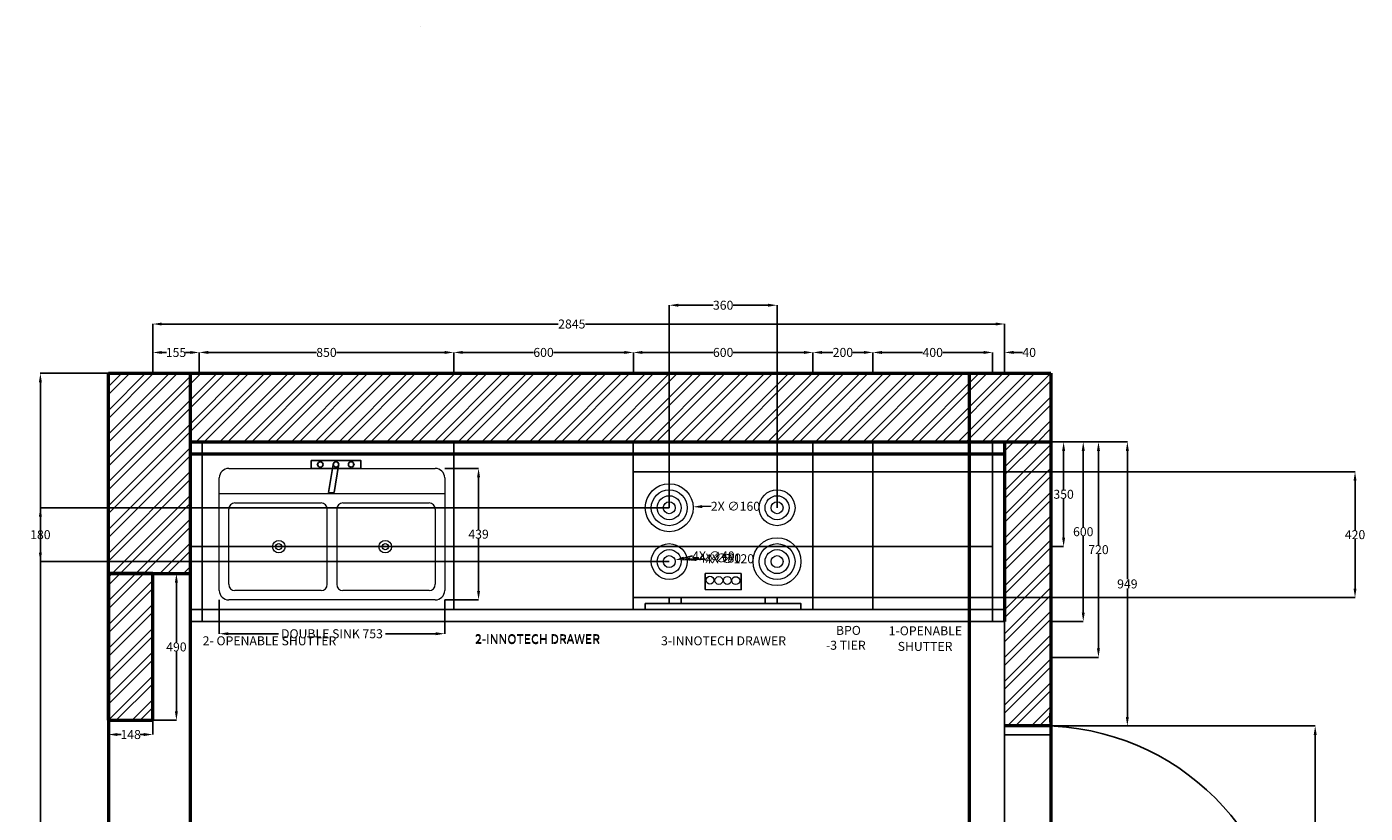
# Model space of a CAD drawing. Units: millimetres. Extents: x 26138 to 44889, y 15820 to 21179.
# Tile 2 of 8: x 26144 to 30614, y 18552 to 21179. Entities that reach past the tile are written whole.
import ezdxf

# ---------------------------------------------------------------- set-up
doc = ezdxf.new("R2010")
doc.units = ezdxf.units.MM
doc.header["$MEASUREMENT"] = 0
doc.header["$PDMODE"] = 3
for name, color, linetype, lineweight in [('A-ANNO-DIMS', 70, 'Continuous', 18), ('A-ANNO-TEXT', 7, 'Continuous', 18), ('A-DOOR', 4, 'Continuous', 25), ('A-EQPM', 8, 'Continuous', 18), ('A-FLOR-FIXT', 8, 'Continuous', 18), ('A-FURN', 26, 'Continuous', 25), ('A-WALL', 1, 'Continuous', 50), ('A-WALL-PATT', 8, 'Continuous', 13)]:
    doc.layers.add(name, color=color, linetype=linetype, lineweight=lineweight)
doc.styles.get("Standard").update_dxf_attribs({"font": 'arial.ttf'})
doc.dimstyles.get("Standard").update_dxf_attribs({"dimtxt": 30, "dimasz": 30, "dimexe": 0.18, "dimexo": 0.0625, "dimgap": 0.09, "dimtad": 0, "dimtih": 1, "dimtoh": 1, "dimdec": 0, "dimzin": 0, "dimdsep": 46, "dimtxsty": 'Standard', "dimcen": 0.09, "dimadec": 0, "dimazin": 0, "dimtfac": 1, "dimtdec": 0, "dimtofl": 0, "dimtmove": 0, "dimatfit": 3, "dimfxl": 1, "dimtolj": 1, "dimtzin": 0, "dimarcsym": 0})
pattern_1 = [(45, (-272.624, -1462.17), (-39.77476, 39.77476), []), (45, (-246.11, -1462.17), (-39.77476, 39.77476), [])]

# ---------------------------------------------------------------- blocks, each defined once
blk = doc.blocks.new('Sink-double - 36 in top')
for p, q in [((-18, -4), (18, -4)), ((-0.75, -18.5), (-0.75, -6.5)), ((0.75, -6.5), (0.75, -18.5))]:
    blk.add_line(p, q)
for points in [[(-16.5, 0), (16.5, 0)], [(-18, -19.5), (-18, -1.5)], [(18, -1.5), (18, -19.5)], [(-15.5, -5.5), (-1.75, -5.5)], [(1.75, -5.5), (15.5, -5.5)], [(-16.5, -18.5), (-16.5, -6.5)], [(16.5, -6.5), (16.5, -18.5)], [(16.5, -21), (-16.5, -21)], [(-1.75, -19.5), (-15.5, -19.5)], [(15.5, -19.5), (1.75, -19.5)]]:
    blk.add_lwpolyline(points)
for centre, radius in [((-8.5, -12.5), 1), ((-8.5, -12.5), 0.5), ((8.5, -12.5), 1), ((8.5, -12.5), 0.5)]:
    blk.add_circle(centre, radius)
for centre, radius, start, end in [((-16.5, -1.5), 1.5, 90, 180), ((16.5, -1.5), 1.5, 0, 90), ((-15.5, -6.5), 1, 90, 180), ((-1.75, -6.5), 1, 0, 90), ((1.75, -6.5), 1, 90, 180), ((15.5, -6.5), 1, 0, 90), ((-15.5, -18.5), 1, 180, 270), ((-1.75, -18.5), 1, 270, 0), ((1.75, -18.5), 1, 180, 270), ((15.5, -18.5), 1, 270, 0), ((-16.5, -19.5), 1.5, 180, 270), ((16.5, -19.5), 1.5, 270, 0)]:
    blk.add_arc(centre, radius, start, end)
blk = doc.blocks.new('*U4')
for p, q in [((0, 0), (0, -6)), ((40, 0), (40, -6))]:
    blk.add_line(p, q)
blk.add_lwpolyline([(0, 0), (0, 40), (1.75, 40), (1.75, 0)], close=True)
blk.add_arc((0, 0), 40, 0, 90)
blk = doc.blocks.new('*D5')
at = {"layer": 'A-ANNO-DIMS', "color": 0, "lineweight": -2, "transparency": 16777216}
for p, q in [((26564.5, 20021.3), (26564.5, 20186.1)), ((26594.5, 20185.9), (27918.7, 20185.9)), ((29379.5, 20185.9), (28009.2, 20185.9)), ((29409.5, 20021.3), (29409.5, 20186.1))]:
    blk.add_line(p, q, dxfattribs=at)
at = {"layer": 'A-ANNO-DIMS', "color": 0, "transparency": 16777216}
for points in [[(26594.5, 20190.9), (26594.5, 20180.9), (26564.5, 20185.9)], [(29379.5, 20190.9), (29379.5, 20180.9), (29409.5, 20185.9)]]:
    blk.add_solid(points, dxfattribs=at)
at = {"layer": 'Defpoints', "color": 0, "transparency": 16777216}
for p in [(29409.5, 20185.9), (26564.5, 20021.2), (29409.5, 20021.2)]:
    blk.add_point(p, dxfattribs=at)
at = {"layer": 'A-ANNO-DIMS', "color": 0, "transparency": 16777216, "insert": (27964, 20185.9), "char_height": 30, "attachment_point": 5}
blk.add_mtext('\\A1;2845', dxfattribs=at)
blk = doc.blocks.new('*D6')
at = {"layer": 'A-ANNO-DIMS', "color": 0, "lineweight": -2, "transparency": 16777216}
for p, q in [((26564.5, 19352.2), (26643.5, 19352.2)), ((26643.3, 19322.2), (26643.3, 19122.6)), ((26643.3, 18892.2), (26643.3, 19091.8)), ((26564.5, 18862.2), (26643.5, 18862.2))]:
    blk.add_line(p, q, dxfattribs=at)
at = {"layer": 'A-ANNO-DIMS', "color": 0, "transparency": 16777216}
for points in [[(26638.3, 19322.2), (26648.3, 19322.2), (26643.3, 19352.2)], [(26638.3, 18892.2), (26648.3, 18892.2), (26643.3, 18862.2)]]:
    blk.add_solid(points, dxfattribs=at)
at = {"layer": 'Defpoints', "color": 0, "transparency": 16777216}
for p in [(26564.5, 19352.2), (26643.3, 19352.2), (26564.5, 18862.2)]:
    blk.add_point(p, dxfattribs=at)
at = {"layer": 'A-ANNO-DIMS', "color": 0, "transparency": 16777216, "insert": (26643.3, 19107.2), "char_height": 30, "attachment_point": 5}
blk.add_mtext('\\A1;490', dxfattribs=at)
blk = doc.blocks.new('*D7')
at = {"layer": 'A-ANNO-DIMS', "color": 0, "lineweight": -2, "transparency": 16777216}
for p, q in [((29564.5, 19792.2), (29606.7, 19792.2)), ((29606.6, 19762.2), (29606.6, 19632.6)), ((29606.6, 19472.2), (29606.6, 19601.8)), ((29564.5, 19442.2), (29606.7, 19442.2))]:
    blk.add_line(p, q, dxfattribs=at)
at = {"layer": 'A-ANNO-DIMS', "color": 0, "transparency": 16777216}
for points in [[(29601.6, 19762.2), (29611.6, 19762.2), (29606.6, 19792.2)], [(29601.6, 19472.2), (29611.6, 19472.2), (29606.6, 19442.2)]]:
    blk.add_solid(points, dxfattribs=at)
at = {"layer": 'Defpoints', "color": 0, "transparency": 16777216}
for p in [(29564.5, 19792.2), (29564.5, 19442.2), (29606.6, 19442.2)]:
    blk.add_point(p, dxfattribs=at)
at = {"layer": 'A-ANNO-DIMS', "color": 0, "transparency": 16777216, "insert": (29606.6, 19617.2), "char_height": 30, "attachment_point": 5}
blk.add_mtext('\\A1;350', dxfattribs=at)
blk = doc.blocks.new('*D8')
at = {"layer": 'A-ANNO-DIMS', "color": 0, "lineweight": -2, "transparency": 16777216}
for p, q in [((29564.5, 19792.2), (29672.4, 19792.2)), ((29672.2, 19762.2), (29672.2, 19507.6)), ((29672.2, 19222.2), (29672.2, 19476.8)), ((29564.5, 19192.2), (29672.4, 19192.2))]:
    blk.add_line(p, q, dxfattribs=at)
at = {"layer": 'A-ANNO-DIMS', "color": 0, "transparency": 16777216}
for points in [[(29667.2, 19762.2), (29677.2, 19762.2), (29672.2, 19792.2)], [(29667.2, 19222.2), (29677.2, 19222.2), (29672.2, 19192.2)]]:
    blk.add_solid(points, dxfattribs=at)
at = {"layer": 'Defpoints', "color": 0, "transparency": 16777216}
for p in [(29564.5, 19792.2), (29564.5, 19192.2), (29672.2, 19192.2)]:
    blk.add_point(p, dxfattribs=at)
at = {"layer": 'A-ANNO-DIMS', "color": 0, "transparency": 16777216, "insert": (29672.2, 19492.2), "char_height": 30, "attachment_point": 5}
blk.add_mtext('\\A1;600', dxfattribs=at)
blk = doc.blocks.new('*D9')
at = {"layer": 'A-ANNO-DIMS', "color": 0, "lineweight": -2, "transparency": 16777216}
for p, q in [((29564.5, 19792.2), (29723.2, 19792.2)), ((29723, 19762.2), (29723, 19447.6)), ((29723, 19102.2), (29723, 19416.8)), ((29564.5, 19072.2), (29723.2, 19072.2))]:
    blk.add_line(p, q, dxfattribs=at)
at = {"layer": 'A-ANNO-DIMS', "color": 0, "transparency": 16777216}
for points in [[(29718, 19762.2), (29728, 19762.2), (29723, 19792.2)], [(29718, 19102.2), (29728, 19102.2), (29723, 19072.2)]]:
    blk.add_solid(points, dxfattribs=at)
at = {"layer": 'Defpoints', "color": 0, "transparency": 16777216}
for p in [(29564.5, 19792.2), (29564.5, 19072.2), (29723, 19072.2)]:
    blk.add_point(p, dxfattribs=at)
at = {"layer": 'A-ANNO-DIMS', "color": 0, "transparency": 16777216, "insert": (29723, 19432.2), "char_height": 30, "attachment_point": 5}
blk.add_mtext('\\A1;720', dxfattribs=at)
blk = doc.blocks.new('*D10')
at = {"layer": 'A-ANNO-DIMS', "color": 0, "lineweight": -2, "transparency": 16777216}
for p, q in [((29564.5, 19792.2), (29819.7, 19792.2)), ((29819.5, 19762.2), (29819.5, 19333.1)), ((29819.5, 18873.2), (29819.5, 19302.3)), ((29564.5, 18843.2), (29819.7, 18843.2))]:
    blk.add_line(p, q, dxfattribs=at)
at = {"layer": 'A-ANNO-DIMS', "color": 0, "transparency": 16777216}
for points in [[(29814.5, 19762.2), (29824.5, 19762.2), (29819.5, 19792.2)], [(29814.5, 18873.2), (29824.5, 18873.2), (29819.5, 18843.2)]]:
    blk.add_solid(points, dxfattribs=at)
at = {"layer": 'Defpoints', "color": 0, "transparency": 16777216}
for p in [(29564.5, 19792.2), (29564.5, 18843.2), (29819.5, 18843.2)]:
    blk.add_point(p, dxfattribs=at)
at = {"layer": 'A-ANNO-DIMS', "color": 0, "transparency": 16777216, "insert": (29819.5, 19317.7), "char_height": 30, "attachment_point": 5}
blk.add_mtext('\\A1;949', dxfattribs=at)
blk = doc.blocks.new('*D11')
at = {"layer": 'A-ANNO-DIMS', "color": 0, "lineweight": -2, "transparency": 16777216}
for p, q in [((26564.5, 20021.3), (26564.5, 20091)), ((26594.5, 20090.8), (26610, 20090.8)), ((26689.5, 20090.8), (26673.9, 20090.8)), ((26719.5, 20021.3), (26719.5, 20091))]:
    blk.add_line(p, q, dxfattribs=at)
at = {"layer": 'A-ANNO-DIMS', "color": 0, "transparency": 16777216}
for points in [[(26594.5, 20095.8), (26594.5, 20085.8), (26564.5, 20090.8)], [(26689.5, 20095.8), (26689.5, 20085.8), (26719.5, 20090.8)]]:
    blk.add_solid(points, dxfattribs=at)
at = {"layer": 'Defpoints', "color": 0, "transparency": 16777216}
for p in [(26719.5, 20090.8), (26564.5, 20021.2), (26719.5, 20021.2)]:
    blk.add_point(p, dxfattribs=at)
at = {"layer": 'A-ANNO-DIMS', "color": 0, "transparency": 16777216, "insert": (26642, 20090.8), "char_height": 30, "attachment_point": 5}
blk.add_mtext('\\A1;155', dxfattribs=at)
blk = doc.blocks.new('*D12')
at = {"layer": 'A-ANNO-DIMS', "color": 0, "lineweight": -2, "transparency": 16777216}
for p, q in [((26719.5, 20021.3), (26719.5, 20091.2)), ((26749.5, 20091), (27111.3, 20091)), ((27539.5, 20091), (27177.7, 20091)), ((27569.5, 20021.3), (27569.5, 20091.2))]:
    blk.add_line(p, q, dxfattribs=at)
at = {"layer": 'A-ANNO-DIMS', "color": 0, "transparency": 16777216}
for points in [[(26749.5, 20096), (26749.5, 20086), (26719.5, 20091)], [(27539.5, 20096), (27539.5, 20086), (27569.5, 20091)]]:
    blk.add_solid(points, dxfattribs=at)
at = {"layer": 'Defpoints', "color": 0, "transparency": 16777216}
for p in [(27569.5, 20091), (26719.5, 20021.2), (27569.5, 20021.2)]:
    blk.add_point(p, dxfattribs=at)
at = {"layer": 'A-ANNO-DIMS', "color": 0, "transparency": 16777216, "insert": (27144.5, 20091), "char_height": 30, "attachment_point": 5}
blk.add_mtext('\\A1;850', dxfattribs=at)
blk = doc.blocks.new('*D13')
at = {"layer": 'A-ANNO-DIMS', "color": 0, "lineweight": -2, "transparency": 16777216}
for p, q in [((27569.5, 20021.3), (27569.5, 20091.2)), ((27599.5, 20091), (27836.2, 20091)), ((28139.5, 20091), (27902.7, 20091)), ((28169.5, 20021.3), (28169.5, 20091.2))]:
    blk.add_line(p, q, dxfattribs=at)
at = {"layer": 'A-ANNO-DIMS', "color": 0, "transparency": 16777216}
for points in [[(27599.5, 20096), (27599.5, 20086), (27569.5, 20091)], [(28139.5, 20096), (28139.5, 20086), (28169.5, 20091)]]:
    blk.add_solid(points, dxfattribs=at)
at = {"layer": 'Defpoints', "color": 0, "transparency": 16777216}
for p in [(28169.5, 20091), (27569.5, 20021.2), (28169.5, 20021.2)]:
    blk.add_point(p, dxfattribs=at)
at = {"layer": 'A-ANNO-DIMS', "color": 0, "transparency": 16777216, "insert": (27869.5, 20091), "char_height": 30, "attachment_point": 5}
blk.add_mtext('\\A1;600', dxfattribs=at)
blk = doc.blocks.new('*D14')
at = {"layer": 'A-ANNO-DIMS', "color": 0, "lineweight": -2, "transparency": 16777216}
for p, q in [((28169.5, 20021.3), (28169.5, 20091.1)), ((28199.5, 20091), (28436.2, 20091)), ((28739.5, 20091), (28502.7, 20091)), ((28769.5, 20021.3), (28769.5, 20091.1))]:
    blk.add_line(p, q, dxfattribs=at)
at = {"layer": 'A-ANNO-DIMS', "color": 0, "transparency": 16777216}
for points in [[(28199.5, 20096), (28199.5, 20086), (28169.5, 20091)], [(28739.5, 20096), (28739.5, 20086), (28769.5, 20091)]]:
    blk.add_solid(points, dxfattribs=at)
at = {"layer": 'Defpoints', "color": 0, "transparency": 16777216}
for p in [(28769.5, 20091), (28169.5, 20021.2), (28769.5, 20021.2)]:
    blk.add_point(p, dxfattribs=at)
at = {"layer": 'A-ANNO-DIMS', "color": 0, "transparency": 16777216, "insert": (28469.5, 20091), "char_height": 30, "attachment_point": 5}
blk.add_mtext('\\A1;600', dxfattribs=at)
blk = doc.blocks.new('*D15')
at = {"layer": 'A-ANNO-DIMS', "color": 0, "lineweight": -2, "transparency": 16777216}
for p, q in [((28769.5, 20021.3), (28769.5, 20091.1)), ((28799.5, 20091), (28836, 20091)), ((28939.5, 20091), (28902.9, 20091)), ((28969.5, 20021.3), (28969.5, 20091.1))]:
    blk.add_line(p, q, dxfattribs=at)
at = {"layer": 'A-ANNO-DIMS', "color": 0, "transparency": 16777216}
for points in [[(28799.5, 20096), (28799.5, 20086), (28769.5, 20091)], [(28939.5, 20096), (28939.5, 20086), (28969.5, 20091)]]:
    blk.add_solid(points, dxfattribs=at)
at = {"layer": 'Defpoints', "color": 0, "transparency": 16777216}
for p in [(28969.5, 20091), (28769.5, 20021.2), (28969.5, 20021.2)]:
    blk.add_point(p, dxfattribs=at)
at = {"layer": 'A-ANNO-DIMS', "color": 0, "transparency": 16777216, "insert": (28869.5, 20091), "char_height": 30, "attachment_point": 5}
blk.add_mtext('\\A1;200', dxfattribs=at)
blk = doc.blocks.new('*D16')
at = {"layer": 'A-ANNO-DIMS', "color": 0, "lineweight": -2, "transparency": 16777216}
for p, q in [((28969.5, 20021.3), (28969.5, 20091.1)), ((28999.5, 20090.9), (29135.7, 20090.9)), ((29339.5, 20090.9), (29203.2, 20090.9)), ((29369.5, 20021.3), (29369.5, 20091.1))]:
    blk.add_line(p, q, dxfattribs=at)
at = {"layer": 'A-ANNO-DIMS', "color": 0, "transparency": 16777216}
for points in [[(28999.5, 20095.9), (28999.5, 20085.9), (28969.5, 20090.9)], [(29339.5, 20095.9), (29339.5, 20085.9), (29369.5, 20090.9)]]:
    blk.add_solid(points, dxfattribs=at)
at = {"layer": 'Defpoints', "color": 0, "transparency": 16777216}
for p in [(29369.5, 20090.9), (28969.5, 20021.2), (29369.5, 20021.2)]:
    blk.add_point(p, dxfattribs=at)
at = {"layer": 'A-ANNO-DIMS', "color": 0, "transparency": 16777216, "insert": (29169.5, 20090.9), "char_height": 30, "attachment_point": 5}
blk.add_mtext('\\A1;400', dxfattribs=at)
blk = doc.blocks.new('*D17')
at = {"layer": 'A-ANNO-DIMS', "color": 0, "lineweight": -2, "transparency": 16777216}
for p, q in [((29339.5, 20091), (29309.5, 20091)), ((29369.5, 20021.3), (29369.5, 20091.1)), ((29409.5, 20021.3), (29409.5, 20091.1)), ((29439.5, 20091), (29469.5, 20091))]:
    blk.add_line(p, q, dxfattribs=at)
at = {"layer": 'A-ANNO-DIMS', "color": 0, "transparency": 16777216}
for points in [[(29339.5, 20096), (29339.5, 20086), (29369.5, 20091)], [(29439.5, 20096), (29439.5, 20086), (29409.5, 20091)]]:
    blk.add_solid(points, dxfattribs=at)
at = {"layer": 'Defpoints', "color": 0, "transparency": 16777216}
for p in [(29409.5, 20091), (29369.5, 20021.2), (29409.5, 20021.2)]:
    blk.add_point(p, dxfattribs=at)
at = {"layer": 'A-ANNO-DIMS', "color": 0, "transparency": 16777216, "insert": (29491.6, 20091), "char_height": 30, "attachment_point": 5}
blk.add_mtext('\\A1;40', dxfattribs=at)
blk = doc.blocks.new('*D19')
at = {"layer": 'A-ANNO-DIMS', "color": 0, "lineweight": -2, "transparency": 16777216}
for p, q in [((29819.6, 18843.2), (30447, 18843.2)), ((30446.9, 18813.2), (30446.9, 18439.3)), ((30446.9, 18053.2), (30446.9, 18408.5)), ((30158.1, 18023.2), (30447, 18023.2))]:
    blk.add_line(p, q, dxfattribs=at)
at = {"layer": 'A-ANNO-DIMS', "color": 0, "transparency": 16777216}
for points in [[(30441.9, 18813.2), (30451.9, 18813.2), (30446.9, 18843.2)], [(30441.9, 18053.2), (30451.9, 18053.2), (30446.9, 18023.2)]]:
    blk.add_solid(points, dxfattribs=at)
at = {"layer": 'Defpoints', "color": 0, "transparency": 16777216}
for p in [(29819.5, 18843.2), (30158.1, 18023.2), (30446.9, 18023.2)]:
    blk.add_point(p, dxfattribs=at)
at = {"layer": 'A-ANNO-DIMS', "color": 0, "transparency": 16777216, "insert": (30446.9, 18423.9), "char_height": 30, "attachment_point": 5}
blk.add_mtext('\\A1;820', dxfattribs=at)
blk = doc.blocks.new('*D120')
at = {"layer": 'A-ANNO-DIMS', "color": 0, "lineweight": -2, "transparency": 16777216}
for p, q in [((26416.5, 18862.1), (26416.5, 18814.4)), ((26564.5, 18862.1), (26564.5, 18814.4)), ((26446.5, 18814.6), (26458.6, 18814.6)), ((26534.5, 18814.6), (26522.3, 18814.6))]:
    blk.add_line(p, q, dxfattribs=at)
at = {"layer": 'A-ANNO-DIMS', "color": 0, "transparency": 16777216}
for points in [[(26446.5, 18819.6), (26446.5, 18809.6), (26416.5, 18814.6)], [(26534.5, 18819.6), (26534.5, 18809.6), (26564.5, 18814.6)]]:
    blk.add_solid(points, dxfattribs=at)
at = {"layer": 'Defpoints', "color": 0, "transparency": 16777216}
for p in [(26416.5, 18862.2), (26564.5, 18862.2), (26564.5, 18814.6)]:
    blk.add_point(p, dxfattribs=at)
at = {"layer": 'A-ANNO-DIMS', "color": 0, "transparency": 16777216, "insert": (26490.5, 18814.6), "char_height": 30, "attachment_point": 5}
blk.add_mtext('\\A1;148', dxfattribs=at)
blk = doc.blocks.new('*D127')
at = {"layer": 'A-ANNO-DIMS', "color": 0, "lineweight": -2, "transparency": 16777216}
for p, q in [((26786.5, 19264.2), (26786.5, 19151.2)), ((27539.5, 19264.2), (27539.5, 19151.2)), ((26816.5, 19151.3), (26983.8, 19151.3)), ((27509.5, 19151.3), (27342.2, 19151.3))]:
    blk.add_line(p, q, dxfattribs=at)
at = {"layer": 'A-ANNO-DIMS', "color": 0, "transparency": 16777216}
for points in [[(26816.5, 19156.3), (26816.5, 19146.3), (26786.5, 19151.3)], [(27509.5, 19156.3), (27509.5, 19146.3), (27539.5, 19151.3)]]:
    blk.add_solid(points, dxfattribs=at)
at = {"layer": 'Defpoints', "color": 0, "transparency": 16777216}
for p in [(26786.5, 19264.3), (27539.5, 19264.3), (27539.5, 19151.3)]:
    blk.add_point(p, dxfattribs=at)
at = {"layer": 'A-ANNO-DIMS', "color": 0, "transparency": 16777216, "insert": (27163, 19151.3), "char_height": 30, "attachment_point": 5}
blk.add_mtext('\\A1;DOUBLE SINK 753', dxfattribs=at)
blk = doc.blocks.new('*D128')
at = {"layer": 'A-ANNO-DIMS', "color": 0, "lineweight": -2, "transparency": 16777216}
for p, q in [((27539.6, 19703.5), (27652.6, 19703.5)), ((27652.5, 19673.5), (27652.5, 19499.3)), ((27652.5, 19294.3), (27652.5, 19468.5)), ((27539.6, 19264.3), (27652.6, 19264.3))]:
    blk.add_line(p, q, dxfattribs=at)
at = {"layer": 'A-ANNO-DIMS', "color": 0, "transparency": 16777216}
for points in [[(27647.5, 19673.5), (27657.5, 19673.5), (27652.5, 19703.5)], [(27647.5, 19294.3), (27657.5, 19294.3), (27652.5, 19264.3)]]:
    blk.add_solid(points, dxfattribs=at)
at = {"layer": 'Defpoints', "color": 0, "transparency": 16777216}
for p in [(27539.5, 19703.5), (27652.5, 19703.5), (27539.5, 19264.3)]:
    blk.add_point(p, dxfattribs=at)
at = {"layer": 'A-ANNO-DIMS', "color": 0, "transparency": 16777216, "insert": (27652.5, 19483.9), "char_height": 30, "attachment_point": 5}
blk.add_mtext('\\A1;439', dxfattribs=at)
blk = doc.blocks.new('*D131')
at = {"layer": 'A-ANNO-DIMS', "color": 0, "lineweight": -2, "transparency": 16777216}
for p, q in [((26416.4, 20021.2), (26188.8, 20021.2)), ((26189, 19991.2), (26189, 18130.6)), ((26189, 16239.2), (26189, 18099.8)), ((26416.4, 16209.2), (26188.8, 16209.2))]:
    blk.add_line(p, q, dxfattribs=at)
at = {"layer": 'A-ANNO-DIMS', "color": 0, "transparency": 16777216}
for points in [[(26184, 19991.2), (26194, 19991.2), (26189, 20021.2)], [(26184, 16239.2), (26194, 16239.2), (26189, 16209.2)]]:
    blk.add_solid(points, dxfattribs=at)
at = {"layer": 'Defpoints', "color": 0, "transparency": 16777216}
for p in [(26416.5, 20021.2), (26189, 16209.2), (26416.5, 16209.2)]:
    blk.add_point(p, dxfattribs=at)
at = {"layer": 'A-ANNO-DIMS', "color": 0, "transparency": 16777216, "insert": (26189, 18115.2), "char_height": 30, "attachment_point": 5}
blk.add_mtext('\\A1;3812', dxfattribs=at)
blk = doc.blocks.new('*D134')
at = {"layer": 'A-ANNO-DIMS', "color": 0, "lineweight": -2, "transparency": 16777216}
for p, q in [((28769.5, 19692.2), (30580.1, 19692.2)), ((30580, 19662.2), (30580, 19497.6)), ((30580, 19302.2), (30580, 19466.8)), ((28769.5, 19272.2), (30580.1, 19272.2))]:
    blk.add_line(p, q, dxfattribs=at)
at = {"layer": 'A-ANNO-DIMS', "color": 0, "transparency": 16777216}
for points in [[(30575, 19662.2), (30585, 19662.2), (30580, 19692.2)], [(30575, 19302.2), (30585, 19302.2), (30580, 19272.2)]]:
    blk.add_solid(points, dxfattribs=at)
at = {"layer": 'Defpoints', "color": 0, "transparency": 16777216}
for p in [(28769.5, 19692.2), (28769.5, 19272.2), (30580, 19272.2)]:
    blk.add_point(p, dxfattribs=at)
at = {"layer": 'A-ANNO-DIMS', "color": 0, "transparency": 16777216, "insert": (30580, 19482.2), "char_height": 30, "attachment_point": 5}
blk.add_mtext('\\A1;420', dxfattribs=at)
blk = doc.blocks.new('*D135')
at = {"layer": 'A-ANNO-DIMS', "color": 0, "lineweight": -2, "transparency": 16777216}
for p, q in [((28289.457271, 19572.265051), (28289.457271, 20248.882635)), ((28319.457271, 20248.702635), (28436.287462, 20248.702635)), ((28619.457271, 20248.702635), (28502.62708, 20248.702635)), ((28649.457271, 19572.265051), (28649.457271, 20248.882635))]:
    blk.add_line(p, q, dxfattribs=at)
at = {"layer": 'A-ANNO-DIMS', "color": 0, "transparency": 16777216}
for points in [[(28319.457271, 20253.702635), (28319.457271, 20243.702635), (28289.457271, 20248.702635)], [(28619.457271, 20253.702635), (28619.457271, 20243.702635), (28649.457271, 20248.702635)]]:
    blk.add_solid(points, dxfattribs=at)
at = {"layer": 'Defpoints', "color": 0, "transparency": 16777216}
for p in [(28649.457271, 20248.702635), (28289.457271, 19572.202551), (28649.457271, 19572.202551)]:
    blk.add_point(p, dxfattribs=at)
at = {"layer": 'A-ANNO-DIMS', "color": 0, "transparency": 16777216, "insert": (28469.457271, 20248.702635), "char_height": 30, "attachment_point": 5}
blk.add_mtext('\\A1;360', dxfattribs=at)
blk = doc.blocks.new('*D136')
at = {"layer": 'A-ANNO-DIMS', "color": 0, "lineweight": -2, "transparency": 16777216}
for p, q in [((28289.4, 19572.2), (26188.8, 19572.2)), ((26189, 19542.2), (26189, 19497.6)), ((26189, 19422.2), (26189, 19466.8)), ((28289.4, 19392.2), (26188.8, 19392.2))]:
    blk.add_line(p, q, dxfattribs=at)
at = {"layer": 'A-ANNO-DIMS', "color": 0, "transparency": 16777216}
for points in [[(26184, 19542.2), (26194, 19542.2), (26189, 19572.2)], [(26184, 19422.2), (26194, 19422.2), (26189, 19392.2)]]:
    blk.add_solid(points, dxfattribs=at)
at = {"layer": 'Defpoints', "color": 0, "transparency": 16777216}
for p in [(28289.5, 19572.2), (26189, 19392.2), (28289.5, 19392.2)]:
    blk.add_point(p, dxfattribs=at)
at = {"layer": 'A-ANNO-DIMS', "color": 0, "transparency": 16777216, "insert": (26189, 19482.2), "char_height": 30, "attachment_point": 5}
blk.add_mtext('\\A1;180', dxfattribs=at)
blk = doc.blocks.new('*D149')
at = {"layer": 'A-ANNO-DIMS', "color": 0, "lineweight": -2, "transparency": 16777216}
for p, q in [((28289.4, 19572.2), (28289.5, 19572.2)), ((28289.5, 19572.1), (28289.5, 19572.3)), ((28429.4, 19577.1), (28399.4, 19576.1))]:
    blk.add_line(p, q, dxfattribs=at)
at = {"layer": 'A-ANNO-DIMS', "color": 0, "transparency": 16777216}
blk.add_solid([(28399.2, 19581.1), (28399.6, 19571.1), (28369.4, 19575)], dxfattribs=at)
at = {"layer": 'Defpoints', "color": 0, "transparency": 16777216}
for p in [(28209.5, 19569.4), (28369.4, 19575)]:
    blk.add_point(p, dxfattribs=at)
at = {"layer": 'A-ANNO-DIMS', "color": 0, "transparency": 16777216, "insert": (28510.6, 19577.1), "char_height": 30, "attachment_point": 5}
blk.add_mtext('\\A1;2X ∅160', dxfattribs=at)
blk = doc.blocks.new('*D150')
at = {"layer": 'A-ANNO-DIMS', "color": 0, "lineweight": -2, "transparency": 16777216}
for p, q in [((28289.4, 19392.2), (28289.5, 19392.2)), ((28289.5, 19392.1), (28289.5, 19392.3)), ((28409.1, 19401.8), (28379.2, 19399.4))]:
    blk.add_line(p, q, dxfattribs=at)
at = {"layer": 'A-ANNO-DIMS', "color": 0, "transparency": 16777216}
blk.add_solid([(28378.8, 19404.4), (28379.6, 19394.4), (28349.3, 19397)], dxfattribs=at)
at = {"layer": 'Defpoints', "color": 0, "transparency": 16777216}
for p in [(28229.7, 19387.4), (28349.3, 19397)]:
    blk.add_point(p, dxfattribs=at)
at = {"layer": 'A-ANNO-DIMS', "color": 0, "transparency": 16777216, "insert": (28490.6, 19401.8), "char_height": 30, "attachment_point": 5}
blk.add_mtext('\\A1;4X ∅120', dxfattribs=at)
blk = doc.blocks.new('*D151')
at = {"layer": 'A-ANNO-DIMS', "color": 0, "lineweight": -2, "transparency": 16777216}
for p, q in [((28388.7, 19404.2), (28358.9, 19400.6)), ((28289.4, 19392.2), (28289.5, 19392.2)), ((28289.5, 19392.1), (28289.5, 19392.3))]:
    blk.add_line(p, q, dxfattribs=at)
at = {"layer": 'A-ANNO-DIMS', "color": 0, "transparency": 16777216}
blk.add_solid([(28358.3, 19405.6), (28359.5, 19395.7), (28329.2, 19397)], dxfattribs=at)
at = {"layer": 'Defpoints', "color": 0, "transparency": 16777216}
for p in [(28249.7, 19387.4), (28329.2, 19397)]:
    blk.add_point(p, dxfattribs=at)
at = {"layer": 'A-ANNO-DIMS', "color": 0, "transparency": 16777216, "insert": (28458.6, 19404.2), "char_height": 30, "attachment_point": 5}
blk.add_mtext('\\A1;4X ∅80', dxfattribs=at)
blk = doc.blocks.new('*D152')
at = {"layer": 'A-ANNO-DIMS', "color": 0, "lineweight": -2, "transparency": 16777216}
for p, q in [((28367.2, 19411.3), (28338, 19404.1)), ((28289.4, 19392.2), (28289.5, 19392.2)), ((28289.5, 19392.1), (28289.5, 19392.3))]:
    blk.add_line(p, q, dxfattribs=at)
at = {"layer": 'A-ANNO-DIMS', "color": 0, "transparency": 16777216}
blk.add_solid([(28336.8, 19409), (28339.2, 19399.3), (28308.9, 19397)], dxfattribs=at)
at = {"layer": 'Defpoints', "color": 0, "transparency": 16777216}
for p in [(28270, 19387.4), (28308.9, 19397)]:
    blk.add_point(p, dxfattribs=at)
at = {"layer": 'A-ANNO-DIMS', "color": 0, "transparency": 16777216, "insert": (28437, 19411.3), "char_height": 30, "attachment_point": 5}
blk.add_mtext('\\A1;4X ∅40', dxfattribs=at)

msp = doc.modelspace()

# ---------------------------------------------------------------- hatches: boundary and pattern name
at = {"layer": 'A-WALL-PATT'}
h = msp.add_hatch(dxfattribs=at)
h.set_pattern_fill('ANSI32', color=256, scale=150)
h.set_pattern_definition(pattern_1)
h.paths.add_polyline_path([(26416.457, 19352.203), (26689.457, 19352.203), (26689.457, 19442.203), (26689.457, 20021.203), (26416.457, 20021.203)])
h = msp.add_hatch(dxfattribs=at)
h.set_pattern_fill('ANSI32', color=256, scale=150)
h.set_pattern_definition(pattern_1)
h.paths.add_polyline_path([(26689.457, 20021.203), (26689.457, 19792.203), (29409.457, 19792.203), (29564.457, 19792.203), (29564.457, 20021.203)])
h = msp.add_hatch(dxfattribs=at)
h.set_pattern_fill('ANSI32', color=256, scale=150)
h.set_pattern_definition(pattern_1)
h.paths.add_polyline_path([(29564.457, 19792.203), (29409.457, 19792.203), (29409.457, 18843.203), (29564.457, 18843.203)])
h = msp.add_hatch(dxfattribs=at)
h.set_pattern_fill('ANSI32', color=256, scale=150)
h.set_pattern_definition(pattern_1)
h.paths.add_polyline_path([(26564.457, 19352.203), (26416.457, 19352.203), (26416.457, 18862.203), (26564.457, 18862.203)])

# ---------------------------------------------------------------- linework, layer by layer
at = {"layer": 'A-EQPM'}
msp.add_line((28529.457, 19352.203), (28409.457, 19352.203), dxfattribs=at)
for centre, radius in [((28289.457, 19572.203), 80), ((28289.457, 19572.203), 60), ((28649.457, 19572.203), 60), ((28289.457, 19572.203), 40), ((28289.457, 19572.203), 20), ((28649.457, 19572.203), 40), ((28649.457, 19572.203), 20), ((28289.457, 19392.203), 60), ((28649.457, 19392.203), 80), ((28649.457, 19392.203), 60), ((28289.457, 19392.203), 40), ((28289.457, 19392.203), 20), ((28649.457, 19392.203), 40), ((28649.457, 19392.203), 20), ((28425.422, 19330.4), 13.132), ((28454.988, 19329.068), 13.132), ((28483.421, 19329.352), 13.132), ((28511.571, 19328.784), 13.132)]:
    msp.add_circle(centre, radius, dxfattribs=at)
at = {"layer": 'A-FURN'}
for p, q in [((26729.457, 19792.203), (26729.457, 19192.203)), ((27569.457, 19792.203), (27569.457, 19232.203)), ((28169.457, 19792.203), (28169.457, 19232.203)), ((28769.457, 19792.203), (28769.457, 19232.203)), ((28969.457, 19792.203), (28969.457, 19232.203)), ((29369.457, 19792.203), (29369.457, 19192.203)), ((29409.457, 19792.203), (29409.457, 16333.203)), ((28169.457, 19692.203), (28769.457, 19692.203)), ((29369.457, 19442.203), (26689.457, 19442.203)), ((28409.457, 19352.203), (28409.457, 19299.311)), ((28529.457, 19298.16), (28529.457, 19352.203)), ((28289.457, 19272.203), (28289.457, 19252.203)), ((28329.457, 19252.203), (28329.457, 19272.203)), ((28409.457, 19299.311), (28529.457, 19298.16)), ((28609.457, 19252.203), (28609.457, 19272.203)), ((28649.457, 19272.203), (28649.457, 19252.203)), ((29409.457, 19232.203), (26689.457, 19232.203)), ((29409.457, 19192.203), (26689.457, 19192.203)), ((29409.457, 18843.203), (29409.457, 18813.203)), ((29564.457, 18813.203), (29564.457, 18843.203)), ((29409.457, 18813.203), (29564.457, 18813.203))]:
    msp.add_line(p, q, dxfattribs=at)
for points in [[(27457.951, 21178.834), (27457.951, 21178.834)], [(27093.077, 19729.8), (27259.452, 19729.8), (27259.452, 19703.524), (27093.077, 19703.524)], [(27115.017, 19716.344), (27113.208, 19716.344), (27113.208, 19717.096), (27115.017, 19717.096)], [(27236.073, 19716.344), (27237.882, 19716.344), (27237.882, 19717.096), (27236.073, 19717.096)], [(28169.457, 19272.203), (28169.457, 19752.203), (28769.457, 19752.203), (28769.457, 19272.203)], [(28209.457, 19232.203), (28209.457, 19252.203), (28729.457, 19252.203), (28729.457, 19232.203)]]:
    msp.add_lwpolyline(points, close=True, dxfattribs=at)
for points in [[(27151.716, 19623.135), (27167.206, 19716.889)], [(27184.845, 19713.747), (27169.874, 19623.135)]]:
    msp.add_lwpolyline(points, dxfattribs=at)
for centre in [(27124.079, 19716.344), (27176.265, 19716.662), (27227.012, 19716.662)]:
    msp.add_circle(centre, 9.062, dxfattribs=at)
msp.add_arc((27160.795, 19657.757), 35.792, 255.305887, 284.694113, dxfattribs=at)
at = {"layer": 'A-WALL'}
for p, q in [((26416.457, 20021.203), (26689.457, 20021.203)), ((26416.457, 18862.203), (26416.457, 20021.203)), ((26689.457, 20021.203), (26689.457, 18862.203)), ((26689.457, 20021.203), (29564.457, 20021.203)), ((29291.457, 20021.203), (29291.457, 16209.203)), ((29564.457, 20021.203), (29564.457, 16209.203)), ((26689.457, 19792.203), (29409.457, 19792.203)), ((29409.457, 19792.203), (29564.457, 19792.203)), ((29409.457, 19792.203), (29409.457, 19192.203)), ((26689.457, 19752.203), (29409.457, 19752.203)), ((26689.457, 19442.203), (26689.457, 16209.203)), ((26416.457, 19352.203), (26416.457, 16209.203)), ((26564.457, 19352.203), (26416.457, 19352.203)), ((26416.457, 19352.203), (26689.457, 19352.203)), ((26564.457, 18862.203), (26564.457, 19352.203)), ((29564.457, 18855.411), (29564.457, 18885.411)), ((26416.457, 18862.203), (26564.457, 18862.203)), ((29564.457, 18843.203), (29409.457, 18843.203))]:
    msp.add_line(p, q, dxfattribs=at)

# ---------------------------------------------------------------- block references
at = {"layer": 'A-DOOR', "xscale": -20.5, "yscale": 20.5, "zscale": 20.5, "rotation": 270}
msp.add_blockref('*U4', (29532.457, 18023.203), dxfattribs=at)
at = {"layer": 'A-FLOR-FIXT', "xscale": 20.9157917650985, "yscale": 20.9157917650985, "zscale": 20.9157917650985}
msp.add_blockref('Sink-double - 36 in top', (27163.023, 19703.524), dxfattribs=at)

# ---------------------------------------------------------------- texts
at = {"layer": 'A-ANNO-TEXT'}
for s, p in [('2- OPENABLE SHUTTER', (26731.13, 19112.745)), ('2-INNOTECH DRAWER', (27640.646, 19119.993)), ('2-INNOTECH DRAWER', (27640.646, 19116.59)), ('3-INNOTECH DRAWER', (28262.142, 19112.745)), ('BPO', (28846.309, 19147.357)), ('1-OPENABLE ', (29022.453, 19146.058)), ('-3 TIER', (28812.85, 19097.802)), ('SHUTTER', (29052.5, 19094.073))]:
    msp.add_text(s, height=30, dxfattribs=at).set_placement(p)

# ---------------------------------------------------------------- dimensions: what is measured, and where the dimension line sits
at = {"layer": 'A-ANNO-DIMS'}
for base, p1, p2, override, picture, middle in [((28649.457, 20248.703), (28289.457, 19572.203), (28649.457, 19572.203), {"dimdec": 0, "dimlfac": 1, "dimrnd": 0, "dimzin": 0, "dimdsep": 46, "dimlunit": 2}, '*D135', (28469.457, 20248.703)), ((26719.457, 20090.832), (26564.457, 20021.203), (26719.457, 20021.203), {"dimclrd": 0, "dimclre": 0, "dimclrt": 0}, '*D11', (26641.957, 20090.832)), ((27569.457, 20091.012), (26719.457, 20021.203), (27569.457, 20021.203), {"dimclrd": 0, "dimclre": 0, "dimclrt": 0}, '*D12', (27144.457, 20091.012)), ((28169.457, 20090.982), (27569.457, 20021.203), (28169.457, 20021.203), {"dimclrd": 0, "dimclre": 0, "dimclrt": 0}, '*D13', (27869.457, 20090.982)), ((28769.457, 20090.952), (28169.457, 20021.203), (28769.457, 20021.203), {"dimclrd": 0, "dimclre": 0, "dimclrt": 0}, '*D14', (28469.457, 20090.952)), ((28969.457, 20090.952), (28769.457, 20021.203), (28969.457, 20021.203), {"dimclrd": 0, "dimclre": 0, "dimclrt": 0}, '*D15', (28869.457, 20090.952)), ((29369.457, 20090.922), (28969.457, 20021.203), (29369.457, 20021.203), {"dimclrd": 0, "dimclre": 0, "dimclrt": 0}, '*D16', (29169.457, 20090.922)), ((29409.457, 20090.952), (29369.457, 20021.203), (29409.457, 20021.203), {"dimclrd": 0, "dimclre": 0, "dimclrt": 0}, '*D17', (29491.587, 20090.952)), ((26564.457, 18814.59), (26416.457, 18862.203), (26564.457, 18862.203), {"dimclrd": 0, "dimclre": 0, "dimclrt": 0}, '*D120', (26490.457, 18814.59))]:
    dim = msp.add_linear_dim(base=base, p1=p1, p2=p2, dimstyle='Standard', override=override, dxfattribs=at)
    dim.commit()
    dim.dimension.update_dxf_attribs({"geometry": picture, "text_midpoint": middle})
dim = msp.add_linear_dim(base=(29409.457, 20185.892), p1=(26564.457, 20021.203), p2=(29409.457, 20021.203), dimstyle='Standard', override={"dimclrd": 0, "dimclre": 0, "dimclrt": 0}, dxfattribs=at)
dim.commit()
dim.dimension.update_dxf_attribs({"geometry": '*D5', "text_midpoint": (27963.972, 20185.892), "dimtype": 160})
for base, p1, p2, override, picture, middle in [((26188.957, 16209.203), (26416.457, 20021.203), (26416.457, 16209.203), {"dimdec": 0, "dimlfac": 1, "dimrnd": 0, "dimzin": 0, "dimdsep": 46, "dimlunit": 2}, '*D131', (26188.957, 18115.203)), ((29606.563, 19442.203), (29564.457, 19792.203), (29564.457, 19442.203), {"dimclrd": 0, "dimclre": 0, "dimclrt": 0}, '*D7', (29606.563, 19617.203)), ((29672.237, 19192.203), (29564.457, 19792.203), (29564.457, 19192.203), {"dimclrd": 0, "dimclre": 0, "dimclrt": 0}, '*D8', (29672.237, 19492.203)), ((29722.985, 19072.203), (29564.457, 19792.203), (29564.457, 19072.203), {"dimclrd": 0, "dimclre": 0, "dimclrt": 0}, '*D9', (29722.985, 19432.203)), ((27652.452, 19703.524), (27539.507, 19264.292), (27539.507, 19703.524), {"dimdec": 0, "dimrnd": 0, "dimzin": 0, "dimlunit": 2}, '*D128', (27652.452, 19483.908)), ((30579.957, 19272.203), (28769.457, 19692.203), (28769.457, 19272.203), {"dimdec": 0, "dimlfac": 1, "dimrnd": 0, "dimzin": 0, "dimdsep": 46, "dimlunit": 2}, '*D134', (30579.957, 19482.203)), ((26188.957, 19392.203), (28289.457, 19572.203), (28289.457, 19392.203), {"dimdec": 0, "dimlfac": 1, "dimrnd": 0, "dimzin": 0, "dimdsep": 46, "dimlunit": 2}, '*D136', (26188.957, 19482.203)), ((26643.306, 19352.203), (26564.457, 18862.203), (26564.457, 19352.203), {"dimclrd": 0, "dimclre": 0, "dimclrt": 0}, '*D6', (26643.306, 19107.203))]:
    dim = msp.add_linear_dim(base=base, p1=p1, p2=p2, angle=90, dimstyle='Standard', override=override, dxfattribs=at)
    dim.commit()
    dim.dimension.update_dxf_attribs({"geometry": picture, "text_midpoint": middle})
for base, p1, p2, picture, middle in [((29819.535, 18843.203), (29564.457, 19792.203), (29564.457, 18843.203), '*D10', (29819.535, 19317.703)), ((30446.851, 18023.203), (29819.535, 18843.203), (30158.053, 18023.203), '*D19', (30446.851, 18423.9))]:
    dim = msp.add_linear_dim(base=base, p1=p1, p2=p2, angle=90, dimstyle='Standard', override={"dimclrd": 0, "dimclre": 0, "dimclrt": 0}, dxfattribs=at)
    dim.commit()
    dim.dimension.update_dxf_attribs({"geometry": picture, "text_midpoint": middle, "dimtype": 160})
for p1, p2, text, picture, middle in [((28209.507, 19569.391), (28369.408, 19575.014), '2X <>', '*D149', (28429.371, 19577.123)), ((28249.748, 19387.385), (28329.166, 19397.02), '4X <>', '*D151', (28388.729, 19404.247)), ((28229.651, 19387.384), (28349.263, 19397.021), '4X <>', '*D150', (28409.07, 19401.84))]:
    dim = msp.add_diameter_dim_2p(p1=p1, p2=p2, text=text, dimstyle='Standard', override={"dimdec": 0, "dimlfac": 1, "dimrnd": 0, "dimzin": 0, "dimdsep": 46, "dimlunit": 2}, dxfattribs=at)
    dim.commit()
    dim.dimension.update_dxf_attribs({"geometry": picture, "text_midpoint": middle, "dimtype": 163})
dim = msp.add_diameter_dim_2p(p1=(28270.034, 19387.434), p2=(28308.881, 19396.971), text='4X <>', dimstyle='Standard', override={"dimdec": 0, "dimlfac": 1, "dimrnd": 0, "dimzin": 0, "dimdsep": 46, "dimlunit": 2}, dxfattribs=at)
dim.commit()
dim.dimension.update_dxf_attribs({"geometry": '*D152', "text_midpoint": (28367.151, 19411.275)})
dim = msp.add_linear_dim(base=(27539.507, 19151.347), p1=(26786.538, 19264.292), p2=(27539.507, 19264.292), text='DOUBLE SINK <>', dimstyle='Standard', override={"dimdec": 0, "dimrnd": 0, "dimzin": 0, "dimlunit": 2}, dxfattribs=at)
dim.commit()
dim.dimension.update_dxf_attribs({"geometry": '*D127', "text_midpoint": (27163.023, 19151.347)})

doc.saveas('drawing.dxf')
